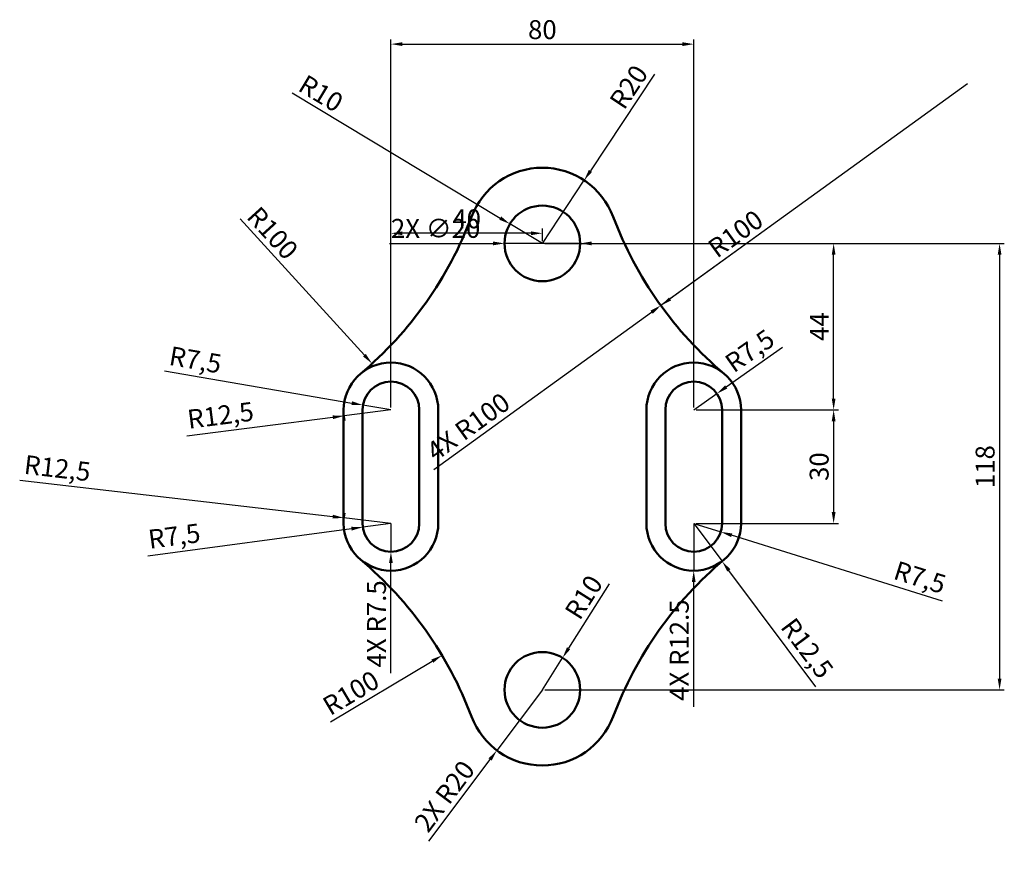
# Model space of a CAD drawing. Units: millimetres. Extents: x 5147 to 5407, y 4365 to 4584.
import ezdxf

# ---------------------------------------------------------------- set-up
doc = ezdxf.new("R2010")
doc.units = ezdxf.units.MM
doc.layers.add('M-DIMS', color=2, linetype='Continuous', lineweight=25)
doc.layers.add('M-OUTL', color=7, linetype='Continuous', lineweight=50)
doc.styles.get("Standard").update_dxf_attribs({"font": 'arial.ttf'})
doc.dimstyles.new('ISO-25', dxfattribs={"dimtxt": 5, "dimasz": 3, "dimexe": 1.25, "dimexo": 0.625, "dimtad": 1, "dimtxsty": 'Standard', "dimcen": 3, "dimadec": 0, "dimazin": 0, "dimtfac": 1, "dimtmove": 0, "dimatfit": 3, "dimfxl": 1, "dimarcsym": 0})

# ---------------------------------------------------------------- blocks, each defined once
blk = doc.blocks.new('*D1')
at = {"layer": 'Defpoints', "color": 0, "transparency": 16777216}
for p in [(5295.89, 4541.39), (5284.84, 4524.72)]:
    blk.add_point(p, dxfattribs=at)
at = {"layer": 'M-DIMS', "color": 0, "lineweight": -2, "transparency": 16777216}
for p, q in [((5314.49, 4569.45), (5297.55, 4543.89)), ((5284.84, 4524.72), (5295.89, 4541.39))]:
    blk.add_line(p, q, dxfattribs=at)
at = {"layer": 'M-DIMS', "color": 0, "transparency": 16777216}
blk.add_solid([(5297.13, 4544.16), (5297.96, 4543.61), (5295.89, 4541.39)], dxfattribs=at)
at = {"layer": 'M-DIMS', "color": 0, "transparency": 16777216, "insert": (5308.2, 4565.71), "char_height": 5, "attachment_point": 5, "rotation": 56.4537}
blk.add_mtext('R20', dxfattribs=at)
blk = doc.blocks.new('*D2')
at = {"layer": 'Defpoints', "color": 0, "transparency": 16777216}
for p in [(5276.27, 4529.87), (5284.84, 4524.72)]:
    blk.add_point(p, dxfattribs=at)
at = {"layer": 'M-DIMS', "color": 0, "lineweight": -2, "transparency": 16777216}
for p, q in [((5218.74, 4564.48), (5273.7, 4531.42)), ((5284.84, 4524.72), (5276.27, 4529.87))]:
    blk.add_line(p, q, dxfattribs=at)
at = {"layer": 'M-DIMS', "color": 0, "transparency": 16777216}
blk.add_solid([(5273.95, 4531.85), (5273.44, 4530.99), (5276.27, 4529.87)], dxfattribs=at)
at = {"layer": 'M-DIMS', "color": 0, "transparency": 16777216, "insert": (5226.02, 4563.81), "char_height": 5, "attachment_point": 5, "rotation": 328.9682}
blk.add_mtext('R10', dxfattribs=at)
blk = doc.blocks.new('*D3')
at = {"layer": 'Defpoints', "color": 0, "transparency": 16777216}
for p in [(5330.97, 4485.03), (5324.84, 4480.72)]:
    blk.add_point(p, dxfattribs=at)
at = {"layer": 'M-DIMS', "color": 0, "lineweight": -2, "transparency": 16777216}
for p, q in [((5348.29, 4497.21), (5333.42, 4486.76)), ((5324.84, 4480.72), (5330.97, 4485.03))]:
    blk.add_line(p, q, dxfattribs=at)
at = {"layer": 'M-DIMS', "color": 0, "transparency": 16777216}
blk.add_solid([(5333.14, 4487.17), (5333.71, 4486.35), (5330.97, 4485.03)], dxfattribs=at)
at = {"layer": 'M-DIMS', "color": 0, "transparency": 16777216, "insert": (5340, 4495.81), "char_height": 5, "attachment_point": 5, "rotation": 35.12}
blk.add_mtext('R7,5', dxfattribs=at)
blk = doc.blocks.new('*D4')
at = {"layer": 'Defpoints', "color": 0, "transparency": 16777216}
for p in [(5232.42, 4452.17), (5244.84, 4450.72)]:
    blk.add_point(p, dxfattribs=at)
at = {"layer": 'M-DIMS', "color": 0, "lineweight": -2, "transparency": 16777216}
for p, q in [((5146.75, 4462.17), (5229.44, 4452.51)), ((5244.84, 4450.72), (5232.42, 4452.17))]:
    blk.add_line(p, q, dxfattribs=at)
blk.add_arc((5244.84, 4450.72), 12.5, 167.61, 177.1352, dxfattribs=at)
at = {"layer": 'M-DIMS', "color": 0, "transparency": 16777216}
blk.add_solid([(5229.5, 4453.01), (5229.38, 4452.02), (5232.42, 4452.17)], dxfattribs=at)
at = {"layer": 'M-DIMS', "color": 0, "transparency": 16777216, "insert": (5156.64, 4464.67), "char_height": 5, "attachment_point": 5, "rotation": 353.3396}
blk.add_mtext('R12,5', dxfattribs=at)
blk = doc.blocks.new('*D5')
at = {"layer": 'Defpoints', "color": 0, "transparency": 16777216}
for p in [(5172.48, 4566.86), (5239.85, 4492.96)]:
    blk.add_point(p, dxfattribs=at)
at = {"layer": 'M-DIMS', "color": 0, "lineweight": -2, "transparency": 16777216}
blk.add_line((5205, 4531.18), (5237.83, 4495.18), dxfattribs=at)
at = {"layer": 'M-DIMS', "color": 0, "transparency": 16777216}
blk.add_solid([(5238.19, 4495.51), (5237.46, 4494.84), (5239.85, 4492.96)], dxfattribs=at)
at = {"layer": 'M-DIMS', "color": 0, "transparency": 16777216, "insert": (5213.1, 4527.02), "char_height": 5, "attachment_point": 5, "rotation": 312.3508}
blk.add_mtext('R100', dxfattribs=at)
blk = doc.blocks.new('*D6')
at = {"layer": 'Defpoints', "color": 0, "transparency": 16777216}
for p in [(5258.34, 4415.84), (5172.48, 4364.57)]:
    blk.add_point(p, dxfattribs=at)
at = {"layer": 'M-DIMS', "color": 0, "lineweight": -2, "transparency": 16777216}
blk.add_line((5228.9, 4398.26), (5255.76, 4414.3), dxfattribs=at)
at = {"layer": 'M-DIMS', "color": 0, "transparency": 16777216}
blk.add_solid([(5255.51, 4414.73), (5256.02, 4413.87), (5258.34, 4415.84)], dxfattribs=at)
at = {"layer": 'M-DIMS', "color": 0, "transparency": 16777216, "insert": (5234.59, 4405.36), "char_height": 5, "attachment_point": 5, "rotation": 30.8392}
blk.add_mtext('R100', dxfattribs=at)
blk = doc.blocks.new('*D7')
at = {"layer": 'Defpoints', "color": 0, "transparency": 16777216}
for p in [(5397.19, 4566.86), (5316.15, 4508.28)]:
    blk.add_point(p, dxfattribs=at)
at = {"layer": 'M-DIMS', "color": 0, "lineweight": -2, "transparency": 16777216}
blk.add_line((5345.03, 4529.16), (5318.58, 4510.04), dxfattribs=at)
at = {"layer": 'M-DIMS', "color": 0, "transparency": 16777216}
blk.add_solid([(5318.29, 4510.44), (5318.87, 4509.63), (5316.15, 4508.28)], dxfattribs=at)
at = {"layer": 'M-DIMS', "color": 0, "transparency": 16777216, "insert": (5336.26, 4526.74), "char_height": 5, "attachment_point": 5, "rotation": 35.8615}
blk.add_mtext('R100', dxfattribs=at)
blk = doc.blocks.new('*D8')
at = {"layer": 'Defpoints', "color": 0, "transparency": 16777216}
for p in [(5324.84, 4450.72), (5331.99, 4448.47)]:
    blk.add_point(p, dxfattribs=at)
at = {"layer": 'M-DIMS', "color": 0, "lineweight": -2, "transparency": 16777216}
for p, q in [((5324.84, 4450.72), (5331.99, 4448.47)), ((5390.57, 4430.12), (5334.85, 4447.58))]:
    blk.add_line(p, q, dxfattribs=at)
at = {"layer": 'M-DIMS', "color": 0, "transparency": 16777216}
blk.add_solid([(5335, 4448.05), (5334.71, 4447.1), (5331.99, 4448.47)], dxfattribs=at)
at = {"layer": 'M-DIMS', "color": 0, "transparency": 16777216, "insert": (5384.41, 4435.84), "char_height": 5, "attachment_point": 5, "rotation": 342.5989}
blk.add_mtext('R7,5', dxfattribs=at)
blk = doc.blocks.new('*D9')
at = {"layer": 'Defpoints', "color": 0, "transparency": 16777216}
for p in [(5324.84, 4450.72), (5332.32, 4440.7)]:
    blk.add_point(p, dxfattribs=at)
at = {"layer": 'M-DIMS', "color": 0, "lineweight": -2, "transparency": 16777216}
for p, q in [((5324.84, 4450.72), (5332.32, 4440.7)), ((5357.1, 4407.54), (5334.11, 4438.3))]:
    blk.add_line(p, q, dxfattribs=at)
at = {"layer": 'M-DIMS', "color": 0, "transparency": 16777216}
blk.add_solid([(5334.51, 4438.6), (5333.71, 4438), (5332.32, 4440.7)], dxfattribs=at)
at = {"layer": 'M-DIMS', "color": 0, "transparency": 16777216, "insert": (5354.3, 4417.35), "char_height": 5, "attachment_point": 5, "rotation": 306.7711}
blk.add_mtext('R12,5', dxfattribs=at)
blk = doc.blocks.new('*D10')
at = {"layer": 'Defpoints', "color": 0, "transparency": 16777216}
for p in [(5237.44, 4481.99), (5244.84, 4480.72)]:
    blk.add_point(p, dxfattribs=at)
at = {"layer": 'M-DIMS', "color": 0, "lineweight": -2, "transparency": 16777216}
for p, q in [((5184.97, 4491.03), (5234.49, 4482.5)), ((5244.84, 4480.72), (5237.44, 4481.99))]:
    blk.add_line(p, q, dxfattribs=at)
at = {"layer": 'M-DIMS', "color": 0, "transparency": 16777216}
blk.add_solid([(5234.57, 4482.99), (5234.4, 4482.01), (5237.44, 4481.99)], dxfattribs=at)
at = {"layer": 'M-DIMS', "color": 0, "transparency": 16777216, "insert": (5193.07, 4493.31), "char_height": 5, "attachment_point": 5, "rotation": 350.2213}
blk.add_mtext('R7,5', dxfattribs=at)
blk = doc.blocks.new('*D11')
at = {"layer": 'Defpoints', "color": 0, "transparency": 16777216}
for p in [(5244.84, 4480.72), (5232.44, 4479.14)]:
    blk.add_point(p, dxfattribs=at)
at = {"layer": 'M-DIMS', "color": 0, "lineweight": -2, "transparency": 16777216}
for p, q in [((5244.84, 4480.72), (5232.44, 4479.14)), ((5190.89, 4473.84), (5229.46, 4478.76))]:
    blk.add_line(p, q, dxfattribs=at)
blk.add_arc((5244.84, 4480.72), 12.5, 182.8648, 192.9926, dxfattribs=at)
at = {"layer": 'M-DIMS', "color": 0, "transparency": 16777216}
blk.add_solid([(5229.4, 4479.25), (5229.52, 4478.26), (5232.44, 4479.14)], dxfattribs=at)
at = {"layer": 'M-DIMS', "color": 0, "transparency": 16777216, "insert": (5199.89, 4478.65), "char_height": 5, "attachment_point": 5, "rotation": 7.2631}
blk.add_mtext('R12,5', dxfattribs=at)
blk = doc.blocks.new('*D12')
at = {"layer": 'Defpoints', "color": 0, "transparency": 16777216}
for p in [(5237.4, 4449.72), (5244.84, 4450.72)]:
    blk.add_point(p, dxfattribs=at)
at = {"layer": 'M-DIMS', "color": 0, "lineweight": -2, "transparency": 16777216}
for p, q in [((5180.63, 4442.14), (5234.43, 4449.33)), ((5244.84, 4450.72), (5237.4, 4449.72))]:
    blk.add_line(p, q, dxfattribs=at)
at = {"layer": 'M-DIMS', "color": 0, "transparency": 16777216}
blk.add_solid([(5234.36, 4449.82), (5234.49, 4448.83), (5237.4, 4449.72)], dxfattribs=at)
at = {"layer": 'M-DIMS', "color": 0, "transparency": 16777216, "insert": (5187.67, 4446.73), "char_height": 5, "attachment_point": 5, "rotation": 7.6122}
blk.add_mtext('R7,5', dxfattribs=at)
blk = doc.blocks.new('*D13')
at = {"layer": 'Defpoints', "color": 0, "transparency": 16777216}
for p in [(5290.18, 4415.17), (5284.84, 4406.72)]:
    blk.add_point(p, dxfattribs=at)
at = {"layer": 'M-DIMS', "color": 0, "lineweight": -2, "transparency": 16777216}
for p, q in [((5302.53, 4434.73), (5291.78, 4417.71)), ((5284.84, 4406.72), (5290.18, 4415.17))]:
    blk.add_line(p, q, dxfattribs=at)
at = {"layer": 'M-DIMS', "color": 0, "transparency": 16777216}
blk.add_solid([(5291.35, 4417.97), (5292.2, 4417.44), (5290.18, 4415.17)], dxfattribs=at)
at = {"layer": 'M-DIMS', "color": 0, "transparency": 16777216, "insert": (5296.32, 4430.86), "char_height": 5, "attachment_point": 5, "rotation": 57.7214}
blk.add_mtext('R10', dxfattribs=at)
blk = doc.blocks.new('*D14')
at = {"layer": 'Defpoints', "color": 0, "transparency": 16777216}
for p in [(5244.84, 4527.39), (5284.84, 4524.72), (5244.84, 4480.72)]:
    blk.add_point(p, dxfattribs=at)
at = {"layer": 'M-DIMS', "color": 0, "lineweight": -2, "transparency": 16777216}
for p, q in [((5244.84, 4481.34), (5244.84, 4528.64)), ((5281.84, 4527.39), (5247.84, 4527.39)), ((5284.84, 4525.34), (5284.84, 4528.64))]:
    blk.add_line(p, q, dxfattribs=at)
at = {"layer": 'M-DIMS', "color": 0, "transparency": 16777216}
for points in [[(5247.84, 4527.89), (5247.84, 4526.89), (5244.84, 4527.39)], [(5281.84, 4527.89), (5281.84, 4526.89), (5284.84, 4527.39)]]:
    blk.add_solid(points, dxfattribs=at)
at = {"layer": 'M-DIMS', "color": 0, "transparency": 16777216, "insert": (5264.84, 4530.56), "char_height": 5, "attachment_point": 5}
blk.add_mtext('40', dxfattribs=at)
blk = doc.blocks.new('*D15')
at = {"layer": 'Defpoints', "color": 0, "transparency": 16777216}
for p in [(5324.84, 4480.72), (5324.84, 4450.72), (5361.8, 4450.72)]:
    blk.add_point(p, dxfattribs=at)
at = {"layer": 'M-DIMS', "color": 0, "lineweight": -2, "transparency": 16777216}
for p, q in [((5325.46, 4480.72), (5363.05, 4480.72)), ((5361.8, 4477.72), (5361.8, 4453.72)), ((5325.46, 4450.72), (5363.05, 4450.72))]:
    blk.add_line(p, q, dxfattribs=at)
at = {"layer": 'M-DIMS', "color": 0, "transparency": 16777216}
for points in [[(5361.3, 4477.72), (5362.3, 4477.72), (5361.8, 4480.72)], [(5361.3, 4453.72), (5362.3, 4453.72), (5361.8, 4450.72)]]:
    blk.add_solid(points, dxfattribs=at)
at = {"layer": 'M-DIMS', "color": 0, "transparency": 16777216, "insert": (5358.62, 4465.72), "char_height": 5, "attachment_point": 5, "rotation": 90}
blk.add_mtext('30', dxfattribs=at)
blk = doc.blocks.new('*D16')
at = {"layer": 'Defpoints', "color": 0, "transparency": 16777216}
for p in [(5284.84, 4524.72), (5361.8, 4524.72), (5324.84, 4480.72)]:
    blk.add_point(p, dxfattribs=at)
at = {"layer": 'M-DIMS', "color": 0, "lineweight": -2, "transparency": 16777216}
for p, q in [((5285.46, 4524.72), (5363.05, 4524.72)), ((5361.8, 4483.72), (5361.8, 4521.72)), ((5325.46, 4480.72), (5363.05, 4480.72))]:
    blk.add_line(p, q, dxfattribs=at)
at = {"layer": 'M-DIMS', "color": 0, "transparency": 16777216}
for points in [[(5361.3, 4521.72), (5362.3, 4521.72), (5361.8, 4524.72)], [(5361.3, 4483.72), (5362.3, 4483.72), (5361.8, 4480.72)]]:
    blk.add_solid(points, dxfattribs=at)
at = {"layer": 'M-DIMS', "color": 0, "transparency": 16777216, "insert": (5358.67, 4502.72), "char_height": 5, "attachment_point": 5, "rotation": 90}
blk.add_mtext('44', dxfattribs=at)
blk = doc.blocks.new('*D17')
at = {"layer": 'Defpoints', "color": 0, "transparency": 16777216}
for p in [(5284.84, 4524.72), (5284.84, 4406.72), (5405.64, 4406.72)]:
    blk.add_point(p, dxfattribs=at)
at = {"layer": 'M-DIMS', "color": 0, "lineweight": -2, "transparency": 16777216}
for p, q in [((5285.46, 4524.72), (5406.89, 4524.72)), ((5405.64, 4521.72), (5405.64, 4409.72)), ((5285.46, 4406.72), (5406.89, 4406.72))]:
    blk.add_line(p, q, dxfattribs=at)
at = {"layer": 'M-DIMS', "color": 0, "transparency": 16777216}
for points in [[(5405.14, 4521.72), (5406.14, 4521.72), (5405.64, 4524.72)], [(5405.14, 4409.72), (5406.14, 4409.72), (5405.64, 4406.72)]]:
    blk.add_solid(points, dxfattribs=at)
at = {"layer": 'M-DIMS', "color": 0, "transparency": 16777216, "insert": (5402.46, 4465.72), "char_height": 5, "attachment_point": 5, "rotation": 90}
blk.add_mtext('118', dxfattribs=at)
blk = doc.blocks.new('*D18')
at = {"layer": 'Defpoints', "color": 0, "transparency": 16777216}
for p in [(5324.84, 4577.39), (5244.84, 4480.72), (5324.84, 4480.72)]:
    blk.add_point(p, dxfattribs=at)
at = {"layer": 'M-DIMS', "color": 0, "lineweight": -2, "transparency": 16777216}
for p, q in [((5244.84, 4481.34), (5244.84, 4578.64)), ((5324.84, 4481.34), (5324.84, 4578.64)), ((5247.84, 4577.39), (5321.84, 4577.39))]:
    blk.add_line(p, q, dxfattribs=at)
at = {"layer": 'M-DIMS', "color": 0, "transparency": 16777216}
for points in [[(5247.84, 4577.89), (5247.84, 4576.89), (5244.84, 4577.39)], [(5321.84, 4577.89), (5321.84, 4576.89), (5324.84, 4577.39)]]:
    blk.add_solid(points, dxfattribs=at)
at = {"layer": 'M-DIMS', "color": 0, "transparency": 16777216, "insert": (5284.84, 4580.57), "char_height": 5, "attachment_point": 5}
blk.add_mtext('80', dxfattribs=at)
blk = doc.blocks.new('MOUNTING-SLOT-15X45-RIM')
for p, q in [((0, 42.5), (0, 12.5)), ((5, 12.5), (5, 42.5)), ((20, 42.5), (20, 12.5)), ((25, 42.5), (25, 12.5))]:
    blk.add_line(p, q)
for centre, radius, start, end in [((12.5, 42.5), 12.5, 0, 180), ((12.5, 42.5), 7.5, 0, 180), ((12.5, 12.5), 12.5, 180, 0), ((12.5, 12.5), 7.5, 180, 0)]:
    blk.add_arc(centre, radius, start, end)
blk = doc.blocks.new('*D20')
at = {"layer": 'Defpoints', "color": 0, "transparency": 16777216}
for p in [(5274.84, 4524.72), (5294.84, 4524.72)]:
    blk.add_point(p, dxfattribs=at)
at = {"layer": 'M-DIMS', "color": 0, "lineweight": -2, "transparency": 16777216}
for p, q in [((5244.44, 4524.72), (5271.84, 4524.72)), ((5294.84, 4524.72), (5274.84, 4524.72)), ((5297.84, 4524.72), (5300.84, 4524.72))]:
    blk.add_line(p, q, dxfattribs=at)
at = {"layer": 'M-DIMS', "color": 0, "transparency": 16777216}
for points in [[(5271.84, 4525.22), (5271.84, 4524.22), (5274.84, 4524.72)], [(5297.84, 4525.22), (5297.84, 4524.22), (5294.84, 4524.72)]]:
    blk.add_solid(points, dxfattribs=at)
at = {"layer": 'M-DIMS', "color": 0, "transparency": 16777216, "insert": (5256.64, 4528.04), "char_height": 5, "attachment_point": 5, "rotation": 359.9987}
blk.add_mtext('2X ∅20', dxfattribs=at)
blk = doc.blocks.new('*D21')
at = {"layer": 'Defpoints', "color": 0, "transparency": 16777216}
for p in [(5284.84, 4406.72), (5272.83, 4390.72)]:
    blk.add_point(p, dxfattribs=at)
at = {"layer": 'M-DIMS', "color": 0, "lineweight": -2, "transparency": 16777216}
for p, q in [((5284.84, 4406.72), (5272.83, 4390.72)), ((5254.83, 4366.71), (5271.03, 4388.32))]:
    blk.add_line(p, q, dxfattribs=at)
at = {"layer": 'M-DIMS', "color": 0, "transparency": 16777216}
blk.add_solid([(5270.63, 4388.62), (5271.43, 4388.02), (5272.83, 4390.72)], dxfattribs=at)
at = {"layer": 'M-DIMS', "color": 0, "transparency": 16777216, "insert": (5259.49, 4378.22), "char_height": 5, "attachment_point": 5, "rotation": 53.1292}
blk.add_mtext('2X R20', dxfattribs=at)
blk = doc.blocks.new('*D22')
at = {"layer": 'Defpoints', "color": 0, "transparency": 16777216}
for p in [(5324.84, 4450.72), (5324.83, 4438.22)]:
    blk.add_point(p, dxfattribs=at)
at = {"layer": 'M-DIMS', "color": 0, "lineweight": -2, "transparency": 16777216}
for p, q in [((5324.84, 4450.72), (5324.83, 4438.22)), ((5324.83, 4402.21), (5324.83, 4435.22))]:
    blk.add_line(p, q, dxfattribs=at)
at = {"layer": 'M-DIMS', "color": 0, "transparency": 16777216}
blk.add_solid([(5324.33, 4435.22), (5325.33, 4435.22), (5324.83, 4438.22)], dxfattribs=at)
at = {"layer": 'M-DIMS', "color": 0, "transparency": 16777216, "insert": (5321.66, 4417.21), "char_height": 5, "attachment_point": 5, "rotation": 89.9989}
blk.add_mtext('4X R12.5', dxfattribs=at)
blk = doc.blocks.new('*D23')
at = {"layer": 'Defpoints', "color": 0, "transparency": 16777216}
for p in [(5244.84, 4450.72), (5244.83, 4443.22)]:
    blk.add_point(p, dxfattribs=at)
at = {"layer": 'M-DIMS', "color": 0, "lineweight": -2, "transparency": 16777216}
for p, q in [((5244.84, 4450.72), (5244.83, 4443.22)), ((5244.83, 4411.1), (5244.83, 4440.22))]:
    blk.add_line(p, q, dxfattribs=at)
at = {"layer": 'M-DIMS', "color": 0, "transparency": 16777216}
blk.add_solid([(5244.33, 4440.22), (5245.33, 4440.22), (5244.83, 4443.22)], dxfattribs=at)
at = {"layer": 'M-DIMS', "color": 0, "transparency": 16777216, "insert": (5241.67, 4424.16), "char_height": 5, "attachment_point": 5, "rotation": 89.9982}
blk.add_mtext('4X R7.5', dxfattribs=at)
blk = doc.blocks.new('*D24')
at = {"layer": 'Defpoints', "color": 0, "transparency": 16777216}
for p in [(5397.19, 4566.86), (5316.13, 4508.3)]:
    blk.add_point(p, dxfattribs=at)
at = {"layer": 'M-DIMS', "color": 0, "lineweight": -2, "transparency": 16777216}
for p, q in [((5397.19, 4566.86), (5316.13, 4508.3)), ((5256.14, 4464.97), (5313.7, 4506.55))]:
    blk.add_line(p, q, dxfattribs=at)
at = {"layer": 'M-DIMS', "color": 0, "transparency": 16777216}
blk.add_solid([(5313.41, 4506.95), (5313.99, 4506.14), (5316.13, 4508.3)], dxfattribs=at)
at = {"layer": 'M-DIMS', "color": 0, "transparency": 16777216, "insert": (5265.63, 4475.74), "char_height": 5, "attachment_point": 5, "rotation": 35.8441}
blk.add_mtext('4X R100', dxfattribs=at)

msp = doc.modelspace()

# ---------------------------------------------------------------- linework, layer by layer
at = {"layer": 'M-OUTL'}
for centre in [(5284.835, 4524.717), (5284.835, 4406.717)]:
    msp.add_circle(centre, 10, dxfattribs=at)
for centre, radius, start, end in [((5284.835, 4524.717), 20, 20.561, 159.439), ((5172.479, 4566.861), 100, 310.0281, 339.439), ((5397.191, 4566.861), 100, 200.561, 229.9719), ((5172.479, 4364.572), 100, 20.561, 49.9719), ((5397.191, 4364.572), 100, 130.0281, 159.439), ((5284.835, 4406.717), 20, 200.561, 339.439)]:
    msp.add_arc(centre, radius, start, end, dxfattribs=at)

# ---------------------------------------------------------------- block references
for p in [(5232.335, 4438.217), (5312.335, 4438.217)]:
    msp.add_blockref('MOUNTING-SLOT-15X45-RIM', p, dxfattribs=at)

# ---------------------------------------------------------------- dimensions: what is measured, and where the dimension line sits
at = {"layer": 'M-DIMS'}
for base, p1, p2, picture, middle in [((5324.835, 4577.391), (5244.835, 4480.717), (5324.835, 4480.717), '*D18', (5284.835, 4580.569)), ((5244.835, 4527.387), (5284.835, 4524.717), (5244.835, 4480.717), '*D14', (5264.835, 4530.565))]:
    dim = msp.add_linear_dim(base=base, p1=p1, p2=p2, dimstyle='ISO-25', override={"dimclrd": 0, "dimclre": 0, "dimclrt": 0}, dxfattribs=at)
    dim.commit()
    dim.dimension.update_dxf_attribs({"geometry": picture, "text_midpoint": middle})
for center, mpoint, picture, middle in [((5284.835, 4524.717), (5295.887, 4541.386), '*D1', (5310.851, 4563.953)), ((5284.835, 4524.717), (5276.266, 4529.872), '*D2', (5224.384, 4561.085)), ((5172.479, 4566.861), (5239.846, 4492.958), '*D5', (5210.75, 4524.877)), ((5397.191, 4566.861), (5316.148, 4508.278), '*D7', (5338.119, 4524.16)), ((5244.835, 4480.717), (5237.444, 4481.991), '*D10', (5192.452, 4489.745)), ((5244.835, 4480.717), (5232.436, 4479.136), '*D11', (5200.345, 4475.047)), ((5244.835, 4450.717), (5232.42, 4452.167), '*D4', (5156.215, 4461.065)), ((5244.835, 4450.717), (5237.401, 4449.723), '*D12', (5188.146, 4443.141)), ((5324.835, 4450.717), (5331.992, 4448.474), '*D8', (5383.326, 4432.386)), ((5324.835, 4450.717), (5332.318, 4440.704), '*D9', (5351.394, 4415.178)), ((5284.835, 4406.717), (5290.176, 4415.171), '*D13', (5299.011, 4429.159)), ((5172.479, 4364.572), (5258.34, 4415.835), '*D6', (5236.224, 4402.631))]:
    dim = msp.add_radius_dim(center=center, mpoint=mpoint, dimstyle='ISO-25', override={"dimclrd": 0, "dimclre": 0, "dimclrt": 0}, dxfattribs=at)
    dim.commit()
    dim.dimension.update_dxf_attribs({"geometry": picture, "text_midpoint": middle, "dimtype": 164})
dim = msp.add_radius_dim(center=(5397.191, 4566.861), mpoint=(5316.13, 4508.303), text='4X <>', dimstyle='ISO-25', override={"dimdec": 0, "dimlfac": 1, "dimrnd": 0, "dimzin": 0, "dimdsep": 46, "dimlunit": 2}, dxfattribs=at)
dim.commit()
dim.dimension.update_dxf_attribs({"geometry": '*D24', "text_midpoint": (5267.493, 4473.168), "dimtype": 164})
dim = msp.add_diameter_dim_2p(p1=(5294.835, 4524.717), p2=(5274.835, 4524.717), text='2X <>', dimstyle='ISO-25', override={"dimdec": 0, "dimlfac": 1, "dimrnd": 0, "dimzin": 0, "dimdsep": 46, "dimlunit": 2}, dxfattribs=at)
dim.commit()
dim.dimension.update_dxf_attribs({"geometry": '*D20', "text_midpoint": (5256.636, 4524.717), "dimtype": 163})
for base, p1, p2, picture, middle in [((5361.798, 4524.717), (5324.835, 4480.717), (5284.835, 4524.717), '*D16', (5358.673, 4502.717)), ((5405.641, 4406.717), (5284.835, 4524.717), (5284.835, 4406.717), '*D17', (5402.463, 4465.717)), ((5361.798, 4450.717), (5324.835, 4480.717), (5324.835, 4450.717), '*D15', (5358.619, 4465.717))]:
    dim = msp.add_linear_dim(base=base, p1=p1, p2=p2, angle=90, dimstyle='ISO-25', override={"dimclrd": 0, "dimclre": 0, "dimclrt": 0}, dxfattribs=at)
    dim.commit()
    dim.dimension.update_dxf_attribs({"geometry": picture, "text_midpoint": middle})
dim = msp.add_radius_dim(center=(5324.835, 4480.717), mpoint=(5330.97, 4485.031), dimstyle='ISO-25', override={"dimclrd": 0, "dimclre": 0, "dimclrt": 0}, dxfattribs=at)
dim.commit()
dim.dimension.update_dxf_attribs({"geometry": '*D3', "text_midpoint": (5340.002, 4495.809)})
for center, mpoint, text, override, picture, middle in [((5244.835, 4450.717), (5244.835, 4443.217), '4X <>', {"dimdec": 1, "dimlfac": 1, "dimrnd": 0, "dimzin": 0, "dimdsep": 46, "dimlunit": 2}, '*D23', (5241.667, 4424.157)), ((5324.835, 4450.717), (5324.835, 4438.217), '4X <>', {"dimdec": 1, "dimlfac": 1, "dimrnd": 0, "dimzin": 0, "dimdsep": 46, "dimlunit": 2}, '*D22', (5321.657, 4417.214)), ((5284.835, 4406.717), (5272.835, 4390.717), '2X <>', {"dimdec": 0, "dimlfac": 1, "dimrnd": 0, "dimzin": 0, "dimdsep": 46, "dimlunit": 2}, '*D21', (5259.49, 4378.22))]:
    dim = msp.add_radius_dim(center=center, mpoint=mpoint, text=text, dimstyle='ISO-25', override=override, dxfattribs=at)
    dim.commit()
    dim.dimension.update_dxf_attribs({"geometry": picture, "text_midpoint": middle})

doc.saveas('drawing.dxf')
